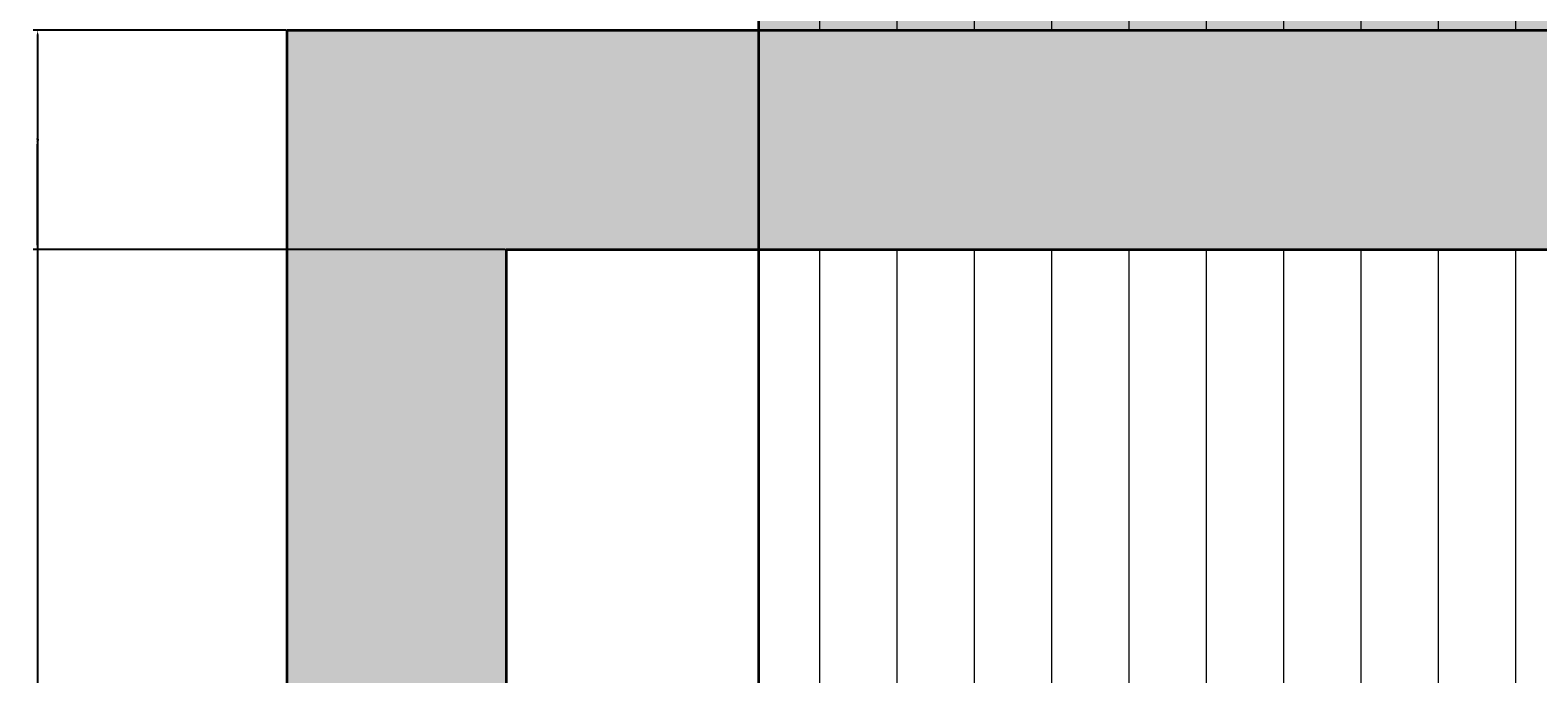
# Model space of a CAD drawing. Units: millimetres. Extents: x 446512 to 447461, y 70395 to 70610.
# Tile 25 of 39: x 446954 to 447016, y 70530 to 70556. Entities that reach past the tile are written whole.
import ezdxf

# ---------------------------------------------------------------- set-up
doc = ezdxf.new("R2010")
doc.units = ezdxf.units.MM
for name, color, linetype, lineweight in [('A-ANNO-DIMS', 2, 'Continuous', 18), ('A-FURN', 7, 'Continuous', 35), ('A-FURN-PATT', 38, 'Continuous', 13)]:
    doc.layers.add(name, color=color, linetype=linetype, lineweight=lineweight)
doc.styles.get("Standard").update_dxf_attribs({"font": 'arial.ttf'})
doc.dimstyles.get("Standard").update_dxf_attribs({"dimtxt": 0.18, "dimasz": 0.18, "dimexe": 0.18, "dimexo": 0.0625, "dimgap": 0.09, "dimtad": 0, "dimtih": 1, "dimtoh": 1, "dimdec": 4, "dimzin": 0, "dimdsep": 46, "dimtxsty": 'Standard', "dimcen": 0.09, "dimadec": 0, "dimazin": 0, "dimtfac": 1, "dimtdec": 4, "dimtofl": 0, "dimtmove": 0, "dimatfit": 3, "dimfxl": 1, "dimtolj": 1, "dimtzin": 0, "dimarcsym": 0})

# ---------------------------------------------------------------- blocks, each defined once
blk = doc.blocks.new('*D54')
at = {"layer": 'A-ANNO-DIMS', "color": 0, "lineweight": -2, "transparency": 16777216}
for p, q in [((446964.107, 70556.451), (446953.739, 70556.451)), ((446953.919, 70556.271), (446953.919, 70499.631)), ((446953.919, 70442.631), (446953.919, 70499.27)), ((446964.107, 70442.451), (446953.739, 70442.451))]:
    blk.add_line(p, q, dxfattribs=at)
at = {"layer": 'A-ANNO-DIMS', "color": 0, "transparency": 16777216}
for points in [[(446953.889, 70556.271), (446953.949, 70556.271), (446953.919, 70556.451)], [(446953.889, 70442.631), (446953.949, 70442.631), (446953.919, 70442.451)]]:
    blk.add_solid(points, dxfattribs=at)
at = {"layer": 'Defpoints', "color": 0, "transparency": 16777216}
for p in [(446953.919, 70556.451), (446964.169, 70556.451), (446964.169, 70442.451)]:
    blk.add_point(p, dxfattribs=at)
at = {"layer": 'A-ANNO-DIMS', "color": 0, "transparency": 16777216, "insert": (446953.919, 70499.451), "char_height": 0.18, "attachment_point": 5}
blk.add_mtext('\\A1;114', dxfattribs=at)
blk = doc.blocks.new('*D59')
at = {"layer": 'A-ANNO-DIMS', "color": 0, "lineweight": -2, "transparency": 16777216}
for p, q in [((446973.107, 70547.451), (446953.739, 70547.451)), ((446953.919, 70547.271), (446953.919, 70515.754)), ((446953.919, 70483.873), (446953.919, 70515.39)), ((446964.107, 70483.693), (446953.739, 70483.693))]:
    blk.add_line(p, q, dxfattribs=at)
at = {"layer": 'A-ANNO-DIMS', "color": 0, "transparency": 16777216}
for points in [[(446953.889, 70547.271), (446953.949, 70547.271), (446953.919, 70547.451)], [(446953.889, 70483.873), (446953.949, 70483.873), (446953.919, 70483.693)]]:
    blk.add_solid(points, dxfattribs=at)
at = {"layer": 'Defpoints', "color": 0, "transparency": 16777216}
for p in [(446953.919, 70547.451), (446973.169, 70547.451), (446964.169, 70483.693)]:
    blk.add_point(p, dxfattribs=at)
at = {"layer": 'A-ANNO-DIMS', "color": 0, "transparency": 16777216, "insert": (446953.919, 70515.572), "char_height": 0.18, "attachment_point": 5}
blk.add_mtext('\\A1;63.76', dxfattribs=at)
blk = doc.blocks.new('*D60')
at = {"layer": 'A-ANNO-DIMS', "color": 0, "lineweight": -2, "transparency": 16777216}
for p, q in [((446964.107, 70556.451), (446953.739, 70556.451)), ((446953.919, 70556.271), (446953.919, 70552.133)), ((446953.919, 70547.631), (446953.919, 70551.769)), ((446973.107, 70547.451), (446953.739, 70547.451))]:
    blk.add_line(p, q, dxfattribs=at)
at = {"layer": 'A-ANNO-DIMS', "color": 0, "transparency": 16777216}
for points in [[(446953.889, 70556.271), (446953.949, 70556.271), (446953.919, 70556.451)], [(446953.889, 70547.631), (446953.949, 70547.631), (446953.919, 70547.451)]]:
    blk.add_solid(points, dxfattribs=at)
at = {"layer": 'Defpoints', "color": 0, "transparency": 16777216}
for p in [(446953.919, 70556.451), (446964.169, 70556.451), (446973.169, 70547.451)]:
    blk.add_point(p, dxfattribs=at)
at = {"layer": 'A-ANNO-DIMS', "color": 0, "transparency": 16777216, "insert": (446953.919, 70551.951), "char_height": 0.18, "attachment_point": 5}
blk.add_mtext('\\A1;9', dxfattribs=at)

msp = doc.modelspace()

# ---------------------------------------------------------------- hatches: boundary and pattern name
at = {"layer": 'A-FURN-PATT'}
h = msp.add_hatch(dxfattribs=at)
h.set_pattern_fill('ANSI31', color=256, angle=45)
h.paths.add_polyline_path([(447044.0961, 70599.7147), (446983.5069, 70599.7147), (446983.5069, 70556.4508), (447030.1693, 70556.4508), (447030.1693, 70442.4508), (446983.5069, 70442.4508), (446983.5069, 70405.3145), (447044.0961, 70405.3145)])
h.paths.add_polyline_path([(447021.1693, 70547.4508), (446983.5069, 70547.4508), (446983.5069, 70451.4508), (447021.1693, 70451.4508)], flags=17)
h = msp.add_hatch(color=256, dxfattribs=at)
h.dxf.hatch_style = 1
h.paths.add_polyline_path([(447021.1693, 70483.6935), (446983.5069, 70483.6935), (446983.5069, 70479.6272), (447021.1693, 70479.6272)], flags=17)
h.paths.add_polyline_path([(447030.1693, 70483.6935), (447021.1693, 70483.6935), (447021.1693, 70479.6272), (447030.1693, 70479.6272)], flags=17)
h.paths.add_polyline_path([(447044.0961, 70599.7147), (446983.5069, 70599.7147), (446983.5069, 70556.4508), (447030.1693, 70556.4508), (447030.1693, 70442.4508), (446983.5069, 70442.4508), (446983.5069, 70405.3145), (447044.0961, 70405.3145)])
h = msp.add_hatch(color=256, dxfattribs=at)
h.dxf.hatch_style = 1
h.paths.add_polyline_path([(446983.5069, 70556.4508), (446964.1693, 70556.4508), (446964.1693, 70442.4508), (446983.5069, 70442.4508), (446983.5069, 70451.4508), (446973.1693, 70451.4508), (446973.1693, 70547.4508), (446983.5069, 70547.4508)])
h.paths.add_polyline_path([(447030.1693, 70556.4508), (446983.5069, 70556.4508), (446983.5069, 70547.4508), (447021.1693, 70547.4508), (447021.1693, 70451.4508), (446983.5069, 70451.4508), (446983.5069, 70442.4508), (447030.1693, 70442.4508)])

# ---------------------------------------------------------------- linework, layer by layer
at = {"layer": 'A-FURN'}
msp.add_line((446983.5069, 70599.7147), (446983.5069, 70405.3145), dxfattribs=at)
for points in [[(447030.1693, 70556.4508), (447030.1693, 70442.4508), (446964.1693, 70442.4508), (446964.1693, 70556.4508)], [(447021.1693, 70547.4508), (447021.1693, 70451.4508), (446973.1693, 70451.4508), (446973.1693, 70547.4508)]]:
    msp.add_lwpolyline(points, close=True, dxfattribs=at)

# ---------------------------------------------------------------- dimensions: what is measured, and where the dimension line sits
at = {"layer": 'A-ANNO-DIMS'}
for base, p1, p2, override, picture, middle in [((446953.9193, 70556.4508), (446964.1693, 70442.4508), (446964.1693, 70556.4508), {"dimdec": 0, "dimlfac": 1, "dimrnd": 0, "dimzin": 0, "dimdsep": 46, "dimlunit": 2}, '*D54', (446953.9193, 70499.4508)), ((446953.9193, 70556.4508), (446973.1693, 70547.4508), (446964.1693, 70556.4508), {"dimdec": 0, "dimlfac": 1, "dimrnd": 0, "dimzin": 0, "dimdsep": 46, "dimlunit": 2}, '*D60', (446953.9193, 70551.9508)), ((446953.9193, 70547.4508), (446964.1693, 70483.6935), (446973.1693, 70547.4508), {"dimdec": 2, "dimlfac": 1, "dimrnd": 0, "dimzin": 0, "dimdsep": 46, "dimlunit": 2}, '*D59', (446953.9193, 70515.5721))]:
    dim = msp.add_linear_dim(base=base, p1=p1, p2=p2, angle=90, dimstyle='Standard', override=override, dxfattribs=at)
    dim.commit()
    dim.dimension.update_dxf_attribs({"geometry": picture, "text_midpoint": middle})

doc.saveas('drawing.dxf')
